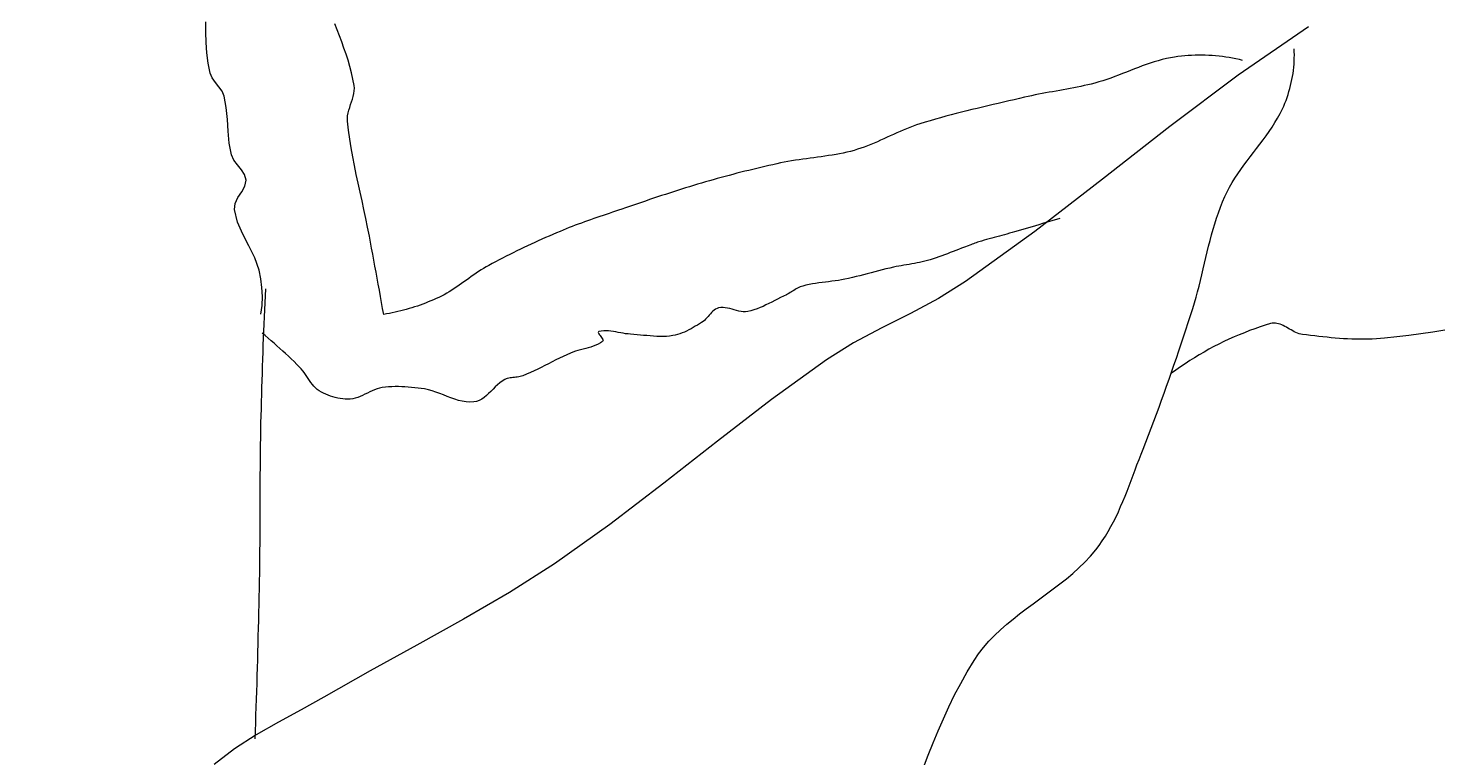
# Model space of a CAD drawing. Units: inches. Extents: x 1441 to 2460, y 1648 to 2683.
# Tile 25 of 35: x 1810 to 1840, y 2253 to 2268. Entities that reach past the tile are written whole.
import ezdxf

# ---------------------------------------------------------------- set-up
doc = ezdxf.new("R2010")
doc.units = ezdxf.units.IN
doc.layers.add('A-ANNO-DIMS', color=2, linetype='Continuous', lineweight=18)
doc.layers.add('A-FURN', color=8, linetype='Continuous', lineweight=15)
doc.styles.get("Standard").update_dxf_attribs({"font": 'arial.ttf'})
doc.dimstyles.get("Standard").update_dxf_attribs({"dimtxt": 0.18, "dimasz": 0.18, "dimexe": 0.18, "dimexo": 0.0625, "dimgap": 0.09, "dimtad": 0, "dimtih": 1, "dimtoh": 1, "dimdec": 4, "dimzin": 0, "dimdsep": 46, "dimtxsty": 'Standard', "dimcen": 0.09, "dimadec": 0, "dimazin": 0, "dimtfac": 1, "dimtdec": 4, "dimtofl": 0, "dimtmove": 0, "dimatfit": 3, "dimfxl": 1, "dimtolj": 1, "dimtzin": 0, "dimarcsym": 0})

# ---------------------------------------------------------------- blocks, each defined once
blk = doc.blocks.new('BED-DOUBLE-PLAN')
for p, q in [((4.673, 72.189), (4.668, 72.41)), ((4.68, 71.967), (4.673, 72.189)), ((7.486, 72.239), (7.436, 72.369)), ((7.535, 72.109), (7.486, 72.239)), ((28.298, 72.301), (26.791, 71.264)), ((4.695, 71.746), (4.68, 71.967)), ((7.583, 71.979), (7.535, 72.109)), ((7.63, 71.848), (7.583, 71.979)), ((4.722, 71.527), (4.695, 71.746)), ((7.675, 71.717), (7.63, 71.848)), ((7.717, 71.585), (7.675, 71.717)), ((7.755, 71.452), (7.717, 71.585)), ((25.076, 71.576), (24.99, 71.55)), ((25.162, 71.599), (25.076, 71.576)), ((25.25, 71.62), (25.162, 71.599)), ((25.337, 71.638), (25.25, 71.62)), ((25.426, 71.654), (25.337, 71.638)), ((25.498, 71.664), (25.426, 71.654)), ((25.571, 71.673), (25.498, 71.664)), ((25.644, 71.68), (25.571, 71.673)), ((25.717, 71.686), (25.644, 71.68)), ((25.79, 71.691), (25.717, 71.686)), ((25.864, 71.694), (25.79, 71.691)), ((25.938, 71.695), (25.864, 71.694)), ((26.011, 71.695), (25.938, 71.695)), ((26.085, 71.694), (26.011, 71.695)), ((26.159, 71.691), (26.085, 71.694)), ((26.233, 71.687), (26.159, 71.691)), ((26.306, 71.681), (26.233, 71.687)), ((26.379, 71.674), (26.306, 71.681)), ((26.453, 71.665), (26.379, 71.674)), ((26.525, 71.655), (26.453, 71.665)), ((26.598, 71.643), (26.525, 71.655)), ((26.67, 71.63), (26.598, 71.643)), ((26.742, 71.616), (26.67, 71.63)), ((26.814, 71.6), (26.742, 71.616)), ((26.885, 71.583), (26.814, 71.6)), ((27.985, 71.502), (27.99, 71.568)), ((27.992, 71.766), (27.99, 71.832)), ((27.99, 71.568), (27.992, 71.634)), ((27.993, 71.7), (27.992, 71.766)), ((27.992, 71.634), (27.993, 71.7)), ((4.765, 71.311), (4.722, 71.527)), ((4.809, 71.206), (4.765, 71.311)), ((7.79, 71.318), (7.755, 71.452)), ((7.821, 71.184), (7.79, 71.318)), ((24.228, 71.268), (24.144, 71.236)), ((24.313, 71.301), (24.228, 71.268)), ((24.397, 71.334), (24.313, 71.301)), ((24.481, 71.366), (24.397, 71.334)), ((24.566, 71.399), (24.481, 71.366)), ((24.65, 71.431), (24.566, 71.399)), ((24.735, 71.463), (24.65, 71.431)), ((24.819, 71.493), (24.735, 71.463)), ((24.904, 71.523), (24.819, 71.493)), ((24.99, 71.55), (24.904, 71.523)), ((27.953, 71.239), (27.964, 71.304)), ((27.964, 71.304), (27.972, 71.37)), ((27.972, 71.37), (27.98, 71.436)), ((27.98, 71.436), (27.985, 71.502)), ((4.876, 71.111), (4.809, 71.206)), ((4.95, 71.019), (4.876, 71.111)), ((5.017, 70.924), (4.95, 71.019)), ((7.846, 71.048), (7.821, 71.184)), ((7.852, 70.989), (7.846, 71.048)), ((7.85, 70.93), (7.852, 70.989)), ((23.116, 70.966), (23.041, 70.952)), ((23.192, 70.98), (23.116, 70.966)), ((23.267, 70.995), (23.192, 70.98)), ((23.342, 71.01), (23.267, 70.995)), ((23.417, 71.025), (23.342, 71.01)), ((23.492, 71.042), (23.417, 71.025)), ((23.567, 71.059), (23.492, 71.042)), ((23.641, 71.077), (23.567, 71.059)), ((23.715, 71.097), (23.641, 71.077)), ((23.802, 71.121), (23.715, 71.097)), ((23.888, 71.147), (23.802, 71.121)), ((23.974, 71.176), (23.888, 71.147)), ((24.059, 71.205), (23.974, 71.176)), ((24.144, 71.236), (24.059, 71.205)), ((26.791, 71.264), (25.327, 70.164)), ((27.877, 70.915), (27.895, 70.979)), ((27.895, 70.979), (27.912, 71.044)), ((27.912, 71.044), (27.927, 71.108)), ((27.927, 71.108), (27.941, 71.173)), ((27.941, 71.173), (27.953, 71.239)), ((5.062, 70.82), (5.017, 70.924)), ((5.108, 70.571), (5.062, 70.82)), ((7.772, 70.636), (7.792, 70.694)), ((7.792, 70.694), (7.811, 70.753)), ((7.811, 70.753), (7.828, 70.812)), ((7.828, 70.812), (7.842, 70.871)), ((7.842, 70.871), (7.85, 70.93)), ((21.648, 70.663), (21.536, 70.636)), ((21.761, 70.689), (21.648, 70.663)), ((21.874, 70.715), (21.761, 70.689)), ((21.987, 70.741), (21.874, 70.715)), ((22.1, 70.767), (21.987, 70.741)), ((22.212, 70.793), (22.1, 70.767)), ((22.287, 70.81), (22.212, 70.793)), ((22.362, 70.827), (22.287, 70.81)), ((22.437, 70.842), (22.362, 70.827)), ((22.512, 70.857), (22.437, 70.842)), ((22.588, 70.871), (22.512, 70.857)), ((22.663, 70.885), (22.588, 70.871)), ((22.739, 70.899), (22.663, 70.885)), ((22.814, 70.912), (22.739, 70.899)), ((22.89, 70.926), (22.814, 70.912)), ((22.965, 70.939), (22.89, 70.926)), ((23.041, 70.952), (22.965, 70.939)), ((27.764, 70.606), (27.789, 70.666)), ((27.789, 70.666), (27.814, 70.727)), ((27.814, 70.727), (27.836, 70.79)), ((27.836, 70.79), (27.858, 70.852)), ((27.858, 70.852), (27.877, 70.915)), ((5.131, 70.318), (5.108, 70.571)), ((7.703, 70.34), (7.708, 70.399)), ((7.708, 70.399), (7.719, 70.459)), ((7.719, 70.459), (7.734, 70.518)), ((7.734, 70.518), (7.752, 70.577)), ((7.752, 70.577), (7.772, 70.636)), ((20.525, 70.385), (20.413, 70.354)), ((20.636, 70.415), (20.525, 70.385)), ((20.748, 70.444), (20.636, 70.415)), ((20.861, 70.473), (20.748, 70.444)), ((20.973, 70.501), (20.861, 70.473)), ((21.085, 70.529), (20.973, 70.501)), ((21.198, 70.556), (21.085, 70.529)), ((21.31, 70.583), (21.198, 70.556)), ((21.423, 70.61), (21.31, 70.583)), ((21.536, 70.636), (21.423, 70.61)), ((27.633, 70.347), (27.687, 70.445)), ((27.687, 70.445), (27.736, 70.546)), ((27.736, 70.546), (27.764, 70.606)), ((5.147, 70.064), (5.131, 70.318)), ((5.17, 69.811), (5.147, 70.064)), ((7.705, 70.28), (7.703, 70.34)), ((7.727, 70.089), (7.705, 70.28)), ((7.754, 69.899), (7.727, 70.089)), ((19.544, 70.06), (19.475, 70.029)), ((19.614, 70.091), (19.544, 70.06)), ((19.684, 70.12), (19.614, 70.091)), ((19.754, 70.148), (19.684, 70.12)), ((19.825, 70.175), (19.754, 70.148)), ((19.897, 70.2), (19.825, 70.175)), ((19.969, 70.223), (19.897, 70.2)), ((20.08, 70.257), (19.969, 70.223)), ((20.191, 70.29), (20.08, 70.257)), ((20.302, 70.323), (20.191, 70.29)), ((20.413, 70.354), (20.302, 70.323)), ((25.327, 70.164), (23.883, 69.037)), ((27.387, 69.97), (27.452, 70.062)), ((27.452, 70.062), (27.515, 70.156)), ((27.515, 70.156), (27.576, 70.251)), ((27.576, 70.251), (27.633, 70.347)), ((5.217, 69.562), (5.17, 69.811)), ((7.784, 69.709), (7.754, 69.899)), ((18.848, 69.753), (18.777, 69.726)), ((18.919, 69.781), (18.848, 69.753)), ((18.989, 69.81), (18.919, 69.781)), ((19.059, 69.841), (18.989, 69.81)), ((19.128, 69.871), (19.059, 69.841)), ((19.197, 69.903), (19.128, 69.871)), ((19.267, 69.935), (19.197, 69.903)), ((19.336, 69.966), (19.267, 69.935)), ((19.405, 69.998), (19.336, 69.966)), ((19.475, 70.029), (19.405, 69.998)), ((27.184, 69.699), (27.253, 69.789)), ((27.253, 69.789), (27.321, 69.879)), ((27.321, 69.879), (27.387, 69.97)), ((5.269, 69.448), (5.217, 69.562)), ((5.347, 69.344), (5.269, 69.448)), ((7.818, 69.519), (7.784, 69.709)), ((7.855, 69.33), (7.818, 69.519)), ((17.38, 69.456), (17.301, 69.444)), ((17.459, 69.467), (17.38, 69.456)), ((17.538, 69.478), (17.459, 69.467)), ((17.618, 69.488), (17.538, 69.478)), ((17.697, 69.499), (17.618, 69.488)), ((17.777, 69.509), (17.697, 69.499)), ((17.856, 69.52), (17.777, 69.509)), ((17.935, 69.531), (17.856, 69.52)), ((18.014, 69.543), (17.935, 69.531)), ((18.093, 69.555), (18.014, 69.543)), ((18.172, 69.569), (18.093, 69.555)), ((18.25, 69.583), (18.172, 69.569)), ((18.329, 69.599), (18.25, 69.583)), ((18.407, 69.617), (18.329, 69.599)), ((18.484, 69.635), (18.407, 69.617)), ((18.561, 69.656), (18.484, 69.635)), ((18.634, 69.678), (18.561, 69.656)), ((18.706, 69.701), (18.634, 69.678)), ((18.777, 69.726), (18.706, 69.701)), ((26.978, 69.429), (27.046, 69.519)), ((27.046, 69.519), (27.115, 69.609)), ((27.115, 69.609), (27.184, 69.699)), ((5.431, 69.242), (5.347, 69.344)), ((5.5, 69.136), (5.431, 69.242)), ((7.893, 69.141), (7.855, 69.33)), ((16.05, 69.164), (15.965, 69.142)), ((16.134, 69.186), (16.05, 69.164)), ((16.219, 69.207), (16.134, 69.186)), ((16.304, 69.228), (16.219, 69.207)), ((16.389, 69.249), (16.304, 69.228)), ((16.474, 69.27), (16.389, 69.249)), ((16.559, 69.29), (16.474, 69.27)), ((16.644, 69.31), (16.559, 69.29)), ((16.73, 69.33), (16.644, 69.31)), ((16.815, 69.349), (16.73, 69.33)), ((16.901, 69.368), (16.815, 69.349)), ((16.986, 69.387), (16.901, 69.368)), ((17.064, 69.403), (16.986, 69.387)), ((17.143, 69.417), (17.064, 69.403)), ((17.222, 69.431), (17.143, 69.417)), ((17.301, 69.444), (17.222, 69.431)), ((26.718, 69.06), (26.78, 69.154)), ((26.78, 69.154), (26.844, 69.246)), ((26.844, 69.246), (26.91, 69.338)), ((26.91, 69.338), (26.978, 69.429)), ((5.44, 68.765), (5.508, 68.888)), ((5.532, 69.019), (5.5, 69.136)), ((5.508, 68.888), (5.532, 69.019)), ((7.934, 68.953), (7.893, 69.141)), ((7.975, 68.764), (7.934, 68.953)), ((14.946, 68.851), (14.86, 68.824)), ((15.032, 68.877), (14.946, 68.851)), ((15.118, 68.903), (15.032, 68.877)), ((15.204, 68.929), (15.118, 68.903)), ((15.29, 68.954), (15.204, 68.929)), ((15.375, 68.979), (15.29, 68.954)), ((15.459, 69.003), (15.375, 68.979)), ((15.543, 69.026), (15.459, 69.003)), ((15.627, 69.05), (15.543, 69.026)), ((15.711, 69.073), (15.627, 69.05)), ((15.796, 69.096), (15.711, 69.073)), ((15.88, 69.119), (15.796, 69.096)), ((15.965, 69.142), (15.88, 69.119)), ((23.883, 69.037), (22.432, 67.918)), ((26.551, 68.769), (26.603, 68.868)), ((26.603, 68.868), (26.659, 68.965)), ((26.659, 68.965), (26.718, 69.06)), ((5.296, 68.52), (5.359, 68.643)), ((5.359, 68.643), (5.44, 68.765)), ((8.017, 68.576), (7.975, 68.764)), ((8.058, 68.388), (8.017, 68.576)), ((14.006, 68.542), (13.921, 68.513)), ((14.091, 68.571), (14.006, 68.542)), ((14.176, 68.6), (14.091, 68.571)), ((14.262, 68.629), (14.176, 68.6)), ((14.347, 68.657), (14.262, 68.629)), ((14.432, 68.686), (14.347, 68.657)), ((14.518, 68.714), (14.432, 68.686)), ((14.603, 68.742), (14.518, 68.714)), ((14.689, 68.769), (14.603, 68.742)), ((14.774, 68.797), (14.689, 68.769)), ((14.86, 68.824), (14.774, 68.797)), ((26.407, 68.437), (26.453, 68.553)), ((26.453, 68.553), (26.503, 68.668)), ((26.503, 68.668), (26.551, 68.769)), ((5.281, 68.391), (5.296, 68.52)), ((5.35, 68.121), (5.281, 68.391)), ((8.098, 68.199), (8.058, 68.388)), ((13.114, 68.24), (13.048, 68.217)), ((13.181, 68.262), (13.114, 68.24)), ((13.247, 68.285), (13.181, 68.262)), ((13.314, 68.307), (13.247, 68.285)), ((13.381, 68.33), (13.314, 68.307)), ((13.447, 68.352), (13.381, 68.33)), ((13.514, 68.375), (13.447, 68.352)), ((13.58, 68.397), (13.514, 68.375)), ((13.665, 68.426), (13.58, 68.397)), ((13.75, 68.455), (13.665, 68.426)), ((13.836, 68.484), (13.75, 68.455)), ((13.921, 68.513), (13.836, 68.484)), ((26.325, 68.203), (26.365, 68.321)), ((26.365, 68.321), (26.407, 68.437)), ((5.463, 67.863), (5.35, 68.121)), ((8.137, 68.01), (8.098, 68.199)), ((8.174, 67.821), (8.137, 68.01)), ((12.324, 67.948), (12.259, 67.921)), ((12.389, 67.974), (12.324, 67.948)), ((12.454, 68.001), (12.389, 67.974)), ((12.519, 68.026), (12.454, 68.001)), ((12.585, 68.051), (12.519, 68.026)), ((12.651, 68.076), (12.585, 68.051)), ((12.717, 68.1), (12.651, 68.076)), ((12.783, 68.124), (12.717, 68.1)), ((12.849, 68.148), (12.783, 68.124)), ((12.915, 68.171), (12.849, 68.148)), ((12.981, 68.194), (12.915, 68.171)), ((13.048, 68.217), (12.981, 68.194)), ((22.073, 67.931), (21.998, 67.909)), ((22.148, 67.953), (22.073, 67.931)), ((22.223, 67.975), (22.148, 67.953)), ((22.297, 67.997), (22.223, 67.975)), ((22.372, 68.019), (22.297, 67.997)), ((22.447, 68.041), (22.372, 68.019)), ((22.521, 68.063), (22.447, 68.041)), ((22.596, 68.086), (22.521, 68.063)), ((22.671, 68.108), (22.596, 68.086)), ((22.745, 68.131), (22.671, 68.108)), ((22.82, 68.154), (22.745, 68.131)), ((22.894, 68.176), (22.82, 68.154)), ((22.969, 68.199), (22.894, 68.176)), ((26.219, 67.844), (26.252, 67.965)), ((26.252, 67.965), (26.287, 68.084)), ((26.287, 68.084), (26.325, 68.203)), ((5.593, 67.609), (5.463, 67.863)), ((8.198, 67.692), (8.174, 67.821)), ((8.222, 67.563), (8.198, 67.692)), ((11.639, 67.646), (11.562, 67.611)), ((11.716, 67.682), (11.639, 67.646)), ((11.793, 67.717), (11.716, 67.682)), ((11.87, 67.752), (11.793, 67.717)), ((11.948, 67.786), (11.87, 67.752)), ((12.025, 67.82), (11.948, 67.786)), ((12.103, 67.854), (12.025, 67.82)), ((12.181, 67.888), (12.103, 67.854)), ((12.259, 67.921), (12.181, 67.888)), ((22.432, 67.918), (20.949, 66.844)), ((21.064, 67.634), (21.036, 67.623)), ((21.092, 67.645), (21.064, 67.634)), ((21.12, 67.655), (21.092, 67.645)), ((21.149, 67.666), (21.12, 67.655)), ((21.177, 67.676), (21.149, 67.666)), ((21.206, 67.686), (21.177, 67.676)), ((21.234, 67.696), (21.206, 67.686)), ((21.263, 67.705), (21.234, 67.696)), ((21.292, 67.714), (21.263, 67.705)), ((21.346, 67.73), (21.292, 67.714)), ((21.4, 67.746), (21.346, 67.73)), ((21.454, 67.761), (21.4, 67.746)), ((21.509, 67.776), (21.454, 67.761)), ((21.563, 67.791), (21.509, 67.776)), ((21.617, 67.806), (21.563, 67.791)), ((21.672, 67.82), (21.617, 67.806)), ((21.726, 67.835), (21.672, 67.82)), ((21.781, 67.849), (21.726, 67.835)), ((21.835, 67.864), (21.781, 67.849)), ((21.89, 67.879), (21.835, 67.864)), ((21.944, 67.894), (21.89, 67.879)), ((21.998, 67.909), (21.944, 67.894)), ((26.156, 67.602), (26.187, 67.724)), ((26.187, 67.724), (26.219, 67.844)), ((5.717, 67.354), (5.593, 67.609)), ((5.81, 67.088), (5.717, 67.354)), ((8.246, 67.434), (8.222, 67.563)), ((8.27, 67.304), (8.246, 67.434)), ((11.03, 67.349), (10.955, 67.31)), ((11.105, 67.388), (11.03, 67.349)), ((11.181, 67.426), (11.105, 67.388)), ((11.257, 67.464), (11.181, 67.426)), ((11.333, 67.501), (11.257, 67.464)), ((11.409, 67.538), (11.333, 67.501)), ((11.486, 67.574), (11.409, 67.538)), ((11.562, 67.611), (11.486, 67.574)), ((20.253, 67.333), (20.191, 67.313)), ((20.315, 67.353), (20.253, 67.333)), ((20.376, 67.375), (20.315, 67.353)), ((20.437, 67.397), (20.376, 67.375)), ((20.498, 67.419), (20.437, 67.397)), ((20.558, 67.442), (20.498, 67.419)), ((20.619, 67.466), (20.558, 67.442)), ((20.679, 67.489), (20.619, 67.466)), ((20.74, 67.513), (20.679, 67.489)), ((20.8, 67.536), (20.74, 67.513)), ((20.861, 67.559), (20.8, 67.536)), ((20.922, 67.581), (20.861, 67.559)), ((20.95, 67.591), (20.922, 67.581)), ((20.979, 67.602), (20.95, 67.591)), ((21.007, 67.612), (20.979, 67.602)), ((21.036, 67.623), (21.007, 67.612)), ((26.069, 67.237), (26.098, 67.359)), ((26.098, 67.359), (26.127, 67.481)), ((26.127, 67.481), (26.156, 67.602)), ((5.849, 66.904), (5.81, 67.088)), ((8.294, 67.175), (8.27, 67.304)), ((8.318, 67.046), (8.294, 67.175)), ((8.341, 66.917), (8.318, 67.046)), ((10.461, 67.024), (10.409, 66.988)), ((10.514, 67.059), (10.461, 67.024)), ((10.567, 67.094), (10.514, 67.059)), ((10.621, 67.127), (10.567, 67.094)), ((10.675, 67.159), (10.621, 67.127)), ((10.731, 67.191), (10.675, 67.159)), ((10.805, 67.231), (10.731, 67.191)), ((10.88, 67.271), (10.805, 67.231)), ((10.955, 67.31), (10.88, 67.271)), ((18.923, 67.033), (18.843, 67.012)), ((19.003, 67.054), (18.923, 67.033)), ((19.083, 67.074), (19.003, 67.054)), ((19.163, 67.095), (19.083, 67.074)), ((19.243, 67.115), (19.163, 67.095)), ((19.324, 67.134), (19.243, 67.115)), ((19.404, 67.153), (19.324, 67.134)), ((19.46, 67.165), (19.404, 67.153)), ((19.515, 67.176), (19.46, 67.165)), ((19.571, 67.186), (19.515, 67.176)), ((19.628, 67.196), (19.571, 67.186)), ((19.684, 67.205), (19.628, 67.196)), ((19.74, 67.214), (19.684, 67.205)), ((19.796, 67.224), (19.74, 67.214)), ((19.852, 67.234), (19.796, 67.224)), ((19.908, 67.244), (19.852, 67.234)), ((19.964, 67.255), (19.908, 67.244)), ((20.019, 67.267), (19.964, 67.255)), ((20.074, 67.28), (20.019, 67.267)), ((20.129, 67.295), (20.074, 67.28)), ((20.191, 67.313), (20.129, 67.295)), ((26.012, 66.993), (26.041, 67.115)), ((26.041, 67.115), (26.069, 67.237)), ((5.873, 66.715), (5.849, 66.904)), ((8.365, 66.787), (8.341, 66.917)), ((8.388, 66.658), (8.365, 66.787)), ((10.045, 66.731), (9.992, 66.695)), ((10.097, 66.767), (10.045, 66.731)), ((10.149, 66.803), (10.097, 66.767)), ((10.201, 66.84), (10.149, 66.803)), ((10.253, 66.877), (10.201, 66.84)), ((10.305, 66.914), (10.253, 66.877)), ((10.357, 66.951), (10.305, 66.914)), ((10.409, 66.988), (10.357, 66.951)), ((17.374, 66.718), (17.347, 66.704)), ((17.402, 66.73), (17.374, 66.718)), ((17.43, 66.741), (17.402, 66.73)), ((17.459, 66.75), (17.43, 66.741)), ((17.527, 66.767), (17.459, 66.75)), ((17.596, 66.782), (17.527, 66.767)), ((17.665, 66.794), (17.596, 66.782)), ((17.734, 66.806), (17.665, 66.794)), ((17.804, 66.816), (17.734, 66.806)), ((17.874, 66.825), (17.804, 66.816)), ((17.944, 66.834), (17.874, 66.825)), ((18.014, 66.843), (17.944, 66.834)), ((18.084, 66.851), (18.014, 66.843)), ((18.154, 66.861), (18.084, 66.851)), ((18.223, 66.871), (18.154, 66.861)), ((18.293, 66.883), (18.223, 66.871)), ((18.362, 66.897), (18.293, 66.883)), ((18.443, 66.914), (18.362, 66.897)), ((18.523, 66.932), (18.443, 66.914)), ((18.603, 66.951), (18.523, 66.932)), ((18.683, 66.971), (18.603, 66.951)), ((18.764, 66.991), (18.683, 66.971)), ((18.843, 67.012), (18.764, 66.991)), ((20.949, 66.844), (20.369, 66.483)), ((25.92, 66.629), (25.952, 66.75)), ((25.952, 66.75), (25.982, 66.871)), ((25.982, 66.871), (26.012, 66.993)), ((5.881, 66.525), (5.873, 66.715)), ((5.874, 66.335), (5.881, 66.525)), ((5.939, 66.39), (5.946, 66.541)), ((5.946, 66.541), (5.953, 66.692)), ((8.412, 66.529), (8.388, 66.658)), ((8.435, 66.399), (8.412, 66.529)), ((9.493, 66.432), (9.436, 66.408)), ((9.55, 66.456), (9.493, 66.432)), ((9.607, 66.481), (9.55, 66.456)), ((9.663, 66.507), (9.607, 66.481)), ((9.72, 66.535), (9.663, 66.507)), ((9.776, 66.564), (9.72, 66.535)), ((9.831, 66.595), (9.776, 66.564)), ((9.886, 66.627), (9.831, 66.595)), ((9.939, 66.661), (9.886, 66.627)), ((9.992, 66.695), (9.939, 66.661)), ((16.859, 66.439), (16.797, 66.407)), ((16.921, 66.471), (16.859, 66.439)), ((16.983, 66.503), (16.921, 66.471)), ((17.045, 66.534), (16.983, 66.503)), ((17.108, 66.564), (17.045, 66.534)), ((17.136, 66.577), (17.108, 66.564)), ((17.163, 66.592), (17.136, 66.577)), ((17.189, 66.608), (17.163, 66.592)), ((17.215, 66.624), (17.189, 66.608)), ((17.241, 66.64), (17.215, 66.624)), ((17.268, 66.657), (17.241, 66.64)), ((17.294, 66.673), (17.268, 66.657)), ((17.32, 66.689), (17.294, 66.673)), ((17.347, 66.704), (17.32, 66.689)), ((20.369, 66.483), (19.765, 66.161)), ((25.852, 66.388), (25.887, 66.508)), ((25.887, 66.508), (25.92, 66.629)), ((5.851, 66.148), (5.874, 66.335)), ((5.926, 66.088), (5.932, 66.239)), ((5.932, 66.239), (5.939, 66.39)), ((8.458, 66.27), (8.435, 66.399)), ((8.481, 66.141), (8.458, 66.27)), ((8.542, 66.151), (8.481, 66.141)), ((8.603, 66.163), (8.542, 66.151)), ((8.664, 66.175), (8.603, 66.163)), ((8.725, 66.188), (8.664, 66.175)), ((8.785, 66.202), (8.725, 66.188)), ((8.845, 66.216), (8.785, 66.202)), ((8.905, 66.232), (8.845, 66.216)), ((8.965, 66.248), (8.905, 66.232)), ((9.025, 66.266), (8.965, 66.248)), ((9.085, 66.284), (9.025, 66.266)), ((9.144, 66.303), (9.085, 66.284)), ((9.203, 66.322), (9.144, 66.303)), ((9.262, 66.342), (9.203, 66.322)), ((9.32, 66.364), (9.262, 66.342)), ((9.378, 66.386), (9.32, 66.364)), ((9.436, 66.408), (9.378, 66.386)), ((15.455, 66.127), (15.43, 66.097)), ((15.481, 66.156), (15.455, 66.127)), ((15.506, 66.183), (15.481, 66.156)), ((15.533, 66.209), (15.506, 66.183)), ((15.561, 66.233), (15.533, 66.209)), ((15.591, 66.253), (15.561, 66.233)), ((15.623, 66.268), (15.591, 66.253)), ((15.658, 66.28), (15.623, 66.268)), ((15.705, 66.287), (15.658, 66.28)), ((15.752, 66.289), (15.705, 66.287)), ((15.8, 66.285), (15.752, 66.289)), ((15.848, 66.277), (15.8, 66.285)), ((15.896, 66.266), (15.848, 66.277)), ((15.945, 66.253), (15.896, 66.266)), ((15.993, 66.239), (15.945, 66.253)), ((16.042, 66.226), (15.993, 66.239)), ((16.09, 66.215), (16.042, 66.226)), ((16.138, 66.206), (16.09, 66.215)), ((16.186, 66.2), (16.138, 66.206)), ((16.234, 66.2), (16.186, 66.2)), ((16.282, 66.206), (16.234, 66.2)), ((16.349, 66.221), (16.282, 66.206)), ((16.415, 66.24), (16.349, 66.221)), ((16.48, 66.263), (16.415, 66.24)), ((16.545, 66.288), (16.48, 66.263)), ((16.609, 66.315), (16.545, 66.288)), ((16.672, 66.344), (16.609, 66.315)), ((16.734, 66.375), (16.672, 66.344)), ((16.797, 66.407), (16.734, 66.375)), ((19.765, 66.161), (19.153, 65.853)), ((25.716, 65.966), (25.765, 66.117)), ((25.765, 66.117), (25.815, 66.269)), ((25.815, 66.269), (25.852, 66.388)), ((5.913, 65.785), (5.92, 65.936)), ((5.92, 65.936), (5.926, 66.088)), ((15.019, 65.81), (14.972, 65.786)), ((15.066, 65.835), (15.019, 65.81)), ((15.112, 65.861), (15.066, 65.835)), ((15.157, 65.887), (15.112, 65.861)), ((15.202, 65.914), (15.157, 65.887)), ((15.247, 65.942), (15.202, 65.914)), ((15.292, 65.969), (15.247, 65.942)), ((15.323, 65.99), (15.292, 65.969)), ((15.351, 66.014), (15.323, 65.99)), ((15.379, 66.04), (15.351, 66.014)), ((15.405, 66.068), (15.379, 66.04)), ((15.43, 66.097), (15.405, 66.068)), ((19.153, 65.853), (18.549, 65.531)), ((25.616, 65.662), (25.666, 65.814)), ((25.666, 65.814), (25.716, 65.966)), ((27.145, 65.835), (27.033, 65.794)), ((27.257, 65.874), (27.145, 65.835)), ((27.37, 65.911), (27.257, 65.874)), ((27.484, 65.946), (27.37, 65.911)), ((27.519, 65.953), (27.484, 65.946)), ((27.553, 65.957), (27.519, 65.953)), ((27.587, 65.955), (27.553, 65.957)), ((27.62, 65.951), (27.587, 65.955)), ((27.654, 65.942), (27.62, 65.951)), ((27.688, 65.931), (27.654, 65.942)), ((27.721, 65.918), (27.688, 65.931)), ((27.755, 65.902), (27.721, 65.918)), ((27.788, 65.885), (27.755, 65.902)), ((27.822, 65.867), (27.788, 65.885)), ((27.855, 65.847), (27.822, 65.867)), ((27.889, 65.828), (27.855, 65.847)), ((27.923, 65.809), (27.889, 65.828)), ((27.957, 65.79), (27.923, 65.809)), ((5.943, 65.687), (5.879, 65.74)), ((5.902, 65.483), (5.908, 65.634)), ((5.908, 65.634), (5.913, 65.785)), ((6.006, 65.633), (5.943, 65.687)), ((6.07, 65.579), (6.006, 65.633)), ((6.133, 65.525), (6.07, 65.579)), ((6.195, 65.47), (6.133, 65.525)), ((13.075, 65.503), (13.024, 65.48)), ((13.123, 65.53), (13.075, 65.503)), ((13.081, 65.766), (13.078, 65.756)), ((13.078, 65.756), (13.081, 65.742)), ((13.093, 65.773), (13.081, 65.766)), ((13.081, 65.742), (13.09, 65.726)), ((13.09, 65.726), (13.103, 65.707)), ((13.144, 65.784), (13.093, 65.773)), ((13.103, 65.707), (13.118, 65.687)), ((13.118, 65.687), (13.135, 65.667)), ((13.169, 65.562), (13.123, 65.53)), ((13.135, 65.667), (13.151, 65.646)), ((13.195, 65.789), (13.144, 65.784)), ((13.151, 65.646), (13.164, 65.626)), ((13.164, 65.626), (13.175, 65.606)), ((13.179, 65.574), (13.169, 65.562)), ((13.175, 65.606), (13.18, 65.589)), ((13.18, 65.589), (13.179, 65.574)), ((13.247, 65.791), (13.195, 65.789)), ((13.298, 65.788), (13.247, 65.791)), ((13.35, 65.783), (13.298, 65.788)), ((13.403, 65.776), (13.35, 65.783)), ((13.455, 65.767), (13.403, 65.776)), ((13.508, 65.757), (13.455, 65.767)), ((13.56, 65.747), (13.508, 65.757)), ((13.613, 65.738), (13.56, 65.747)), ((13.665, 65.729), (13.613, 65.738)), ((13.718, 65.723), (13.665, 65.729)), ((13.77, 65.718), (13.718, 65.723)), ((13.84, 65.714), (13.77, 65.718)), ((13.91, 65.708), (13.84, 65.714)), ((13.98, 65.701), (13.91, 65.708)), ((14.05, 65.694), (13.98, 65.701)), ((14.12, 65.688), (14.05, 65.694)), ((14.19, 65.681), (14.12, 65.688)), ((14.26, 65.676), (14.19, 65.681)), ((14.33, 65.672), (14.26, 65.676)), ((14.399, 65.669), (14.33, 65.672)), ((14.469, 65.669), (14.399, 65.669)), ((14.539, 65.672), (14.469, 65.669)), ((14.608, 65.678), (14.539, 65.672)), ((14.677, 65.687), (14.608, 65.678)), ((14.728, 65.697), (14.677, 65.687)), ((14.778, 65.71), (14.728, 65.697)), ((14.828, 65.726), (14.778, 65.71)), ((14.876, 65.744), (14.828, 65.726)), ((14.924, 65.764), (14.876, 65.744)), ((14.972, 65.786), (14.924, 65.764)), ((18.549, 65.531), (17.968, 65.172)), ((25.515, 65.359), (25.566, 65.51)), ((25.566, 65.51), (25.616, 65.662)), ((26.375, 65.506), (26.269, 65.452)), ((26.483, 65.559), (26.375, 65.506)), ((26.591, 65.61), (26.483, 65.559)), ((26.7, 65.659), (26.591, 65.61)), ((26.81, 65.706), (26.7, 65.659)), ((26.921, 65.751), (26.81, 65.706)), ((27.033, 65.794), (26.921, 65.751)), ((27.991, 65.772), (27.957, 65.79)), ((28.025, 65.756), (27.991, 65.772)), ((28.06, 65.741), (28.025, 65.756)), ((28.094, 65.729), (28.06, 65.741)), ((28.13, 65.72), (28.094, 65.729)), ((28.165, 65.713), (28.13, 65.72)), ((28.253, 65.702), (28.165, 65.713)), ((28.34, 65.691), (28.253, 65.702)), ((28.428, 65.681), (28.34, 65.691)), ((28.516, 65.67), (28.428, 65.681)), ((28.604, 65.661), (28.516, 65.67)), ((28.692, 65.652), (28.604, 65.661)), ((28.78, 65.643), (28.692, 65.652)), ((28.869, 65.635), (28.78, 65.643)), ((28.957, 65.628), (28.869, 65.635)), ((29.045, 65.622), (28.957, 65.628)), ((29.133, 65.617), (29.045, 65.622)), ((29.222, 65.613), (29.133, 65.617)), ((29.31, 65.611), (29.222, 65.613)), ((29.398, 65.609), (29.31, 65.611)), ((29.487, 65.609), (29.398, 65.609)), ((29.575, 65.61), (29.487, 65.609)), ((29.663, 65.613), (29.575, 65.61)), ((29.751, 65.618), (29.663, 65.613)), ((29.839, 65.624), (29.751, 65.618)), ((29.927, 65.632), (29.839, 65.624)), ((30.186, 65.66), (29.927, 65.632)), ((30.444, 65.692), (30.186, 65.66)), ((30.702, 65.727), (30.444, 65.692)), ((30.96, 65.765), (30.702, 65.727)), ((31.218, 65.805), (30.96, 65.765)), ((5.891, 65.181), (5.896, 65.332)), ((5.896, 65.332), (5.902, 65.483)), ((6.257, 65.414), (6.195, 65.47)), ((6.319, 65.358), (6.257, 65.414)), ((6.38, 65.302), (6.319, 65.358)), ((6.44, 65.245), (6.38, 65.302)), ((6.501, 65.188), (6.44, 65.245)), ((12.246, 65.204), (12.168, 65.166)), ((12.324, 65.242), (12.246, 65.204)), ((12.403, 65.279), (12.324, 65.242)), ((12.482, 65.314), (12.403, 65.279)), ((12.535, 65.335), (12.482, 65.314)), ((12.588, 65.353), (12.535, 65.335)), ((12.643, 65.369), (12.588, 65.353)), ((12.698, 65.384), (12.643, 65.369)), ((12.754, 65.398), (12.698, 65.384)), ((12.809, 65.412), (12.754, 65.398)), ((12.864, 65.426), (12.809, 65.412)), ((12.919, 65.442), (12.864, 65.426)), ((12.972, 65.46), (12.919, 65.442)), ((13.024, 65.48), (12.972, 65.46)), ((25.413, 65.056), (25.464, 65.207)), ((25.464, 65.207), (25.515, 65.359)), ((25.853, 65.215), (25.752, 65.152)), ((25.955, 65.277), (25.853, 65.215)), ((26.059, 65.337), (25.955, 65.277)), ((26.163, 65.395), (26.059, 65.337)), ((26.269, 65.452), (26.163, 65.395)), ((5.881, 64.878), (5.886, 65.029)), ((5.886, 65.029), (5.891, 65.181)), ((6.56, 65.13), (6.501, 65.188)), ((6.619, 65.071), (6.56, 65.13)), ((6.678, 65.013), (6.619, 65.071)), ((6.713, 64.975), (6.678, 65.013)), ((6.745, 64.936), (6.713, 64.975)), ((6.776, 64.895), (6.745, 64.936)), ((11.702, 64.932), (11.623, 64.896)), ((11.78, 64.97), (11.702, 64.932)), ((11.858, 65.008), (11.78, 64.97)), ((11.935, 65.048), (11.858, 65.008)), ((12.013, 65.087), (11.935, 65.048)), ((12.09, 65.127), (12.013, 65.087)), ((12.168, 65.166), (12.09, 65.127)), ((17.968, 65.172), (16.787, 64.32)), ((25.308, 64.754), (25.361, 64.905)), ((25.456, 64.951), (25.36, 64.881)), ((25.361, 64.905), (25.413, 65.056)), ((25.553, 65.02), (25.456, 64.951)), ((25.652, 65.087), (25.553, 65.02)), ((25.752, 65.152), (25.652, 65.087)), ((5.872, 64.576), (5.876, 64.727)), ((5.876, 64.727), (5.881, 64.878)), ((6.805, 64.853), (6.776, 64.895)), ((6.834, 64.81), (6.805, 64.853)), ((6.863, 64.767), (6.834, 64.81)), ((6.892, 64.724), (6.863, 64.767)), ((6.922, 64.683), (6.892, 64.724)), ((6.953, 64.643), (6.922, 64.683)), ((6.985, 64.605), (6.953, 64.643)), ((7.021, 64.569), (6.985, 64.605)), ((8.657, 64.594), (8.587, 64.59)), ((8.727, 64.596), (8.657, 64.594)), ((8.797, 64.596), (8.727, 64.596)), ((8.867, 64.594), (8.797, 64.596)), ((8.937, 64.591), (8.867, 64.594)), ((10.919, 64.633), (10.871, 64.588)), ((10.969, 64.676), (10.919, 64.633)), ((11.02, 64.714), (10.969, 64.676)), ((11.074, 64.746), (11.02, 64.714)), ((11.102, 64.759), (11.074, 64.746)), ((11.13, 64.769), (11.102, 64.759)), ((11.16, 64.777), (11.13, 64.769)), ((11.19, 64.782), (11.16, 64.777)), ((11.22, 64.787), (11.19, 64.782)), ((11.251, 64.79), (11.22, 64.787)), ((11.282, 64.793), (11.251, 64.79)), ((11.313, 64.796), (11.282, 64.793)), ((11.344, 64.799), (11.313, 64.796)), ((11.375, 64.803), (11.344, 64.799)), ((11.405, 64.809), (11.375, 64.803)), ((11.435, 64.817), (11.405, 64.809)), ((11.463, 64.827), (11.435, 64.817)), ((11.544, 64.86), (11.463, 64.827)), ((11.623, 64.896), (11.544, 64.86)), ((25.202, 64.453), (25.256, 64.603)), ((25.256, 64.603), (25.308, 64.754)), ((5.863, 64.273), (5.868, 64.425)), ((5.868, 64.425), (5.872, 64.576)), ((7.058, 64.536), (7.021, 64.569)), ((7.099, 64.507), (7.058, 64.536)), ((7.145, 64.48), (7.099, 64.507)), ((7.192, 64.455), (7.145, 64.48)), ((7.24, 64.432), (7.192, 64.455)), ((7.289, 64.411), (7.24, 64.432)), ((7.34, 64.392), (7.289, 64.411)), ((7.391, 64.375), (7.34, 64.392)), ((7.443, 64.361), (7.391, 64.375)), ((7.496, 64.349), (7.443, 64.361)), ((7.549, 64.339), (7.496, 64.349)), ((7.602, 64.333), (7.549, 64.339)), ((7.655, 64.328), (7.602, 64.333)), ((7.708, 64.327), (7.655, 64.328)), ((7.761, 64.328), (7.708, 64.327)), ((7.817, 64.334), (7.761, 64.328)), ((7.871, 64.346), (7.817, 64.334)), ((7.924, 64.363), (7.871, 64.346)), ((7.976, 64.383), (7.924, 64.363)), ((8.028, 64.406), (7.976, 64.383)), ((8.08, 64.431), (8.028, 64.406)), ((8.131, 64.457), (8.08, 64.431)), ((8.183, 64.483), (8.131, 64.457)), ((8.234, 64.508), (8.183, 64.483)), ((8.286, 64.53), (8.234, 64.508)), ((8.339, 64.55), (8.286, 64.53)), ((8.393, 64.565), (8.339, 64.55)), ((8.448, 64.576), (8.393, 64.565)), ((8.518, 64.584), (8.448, 64.576)), ((8.587, 64.59), (8.518, 64.584)), ((9.007, 64.586), (8.937, 64.591)), ((9.077, 64.58), (9.007, 64.586)), ((9.147, 64.573), (9.077, 64.58)), ((9.217, 64.564), (9.147, 64.573)), ((9.286, 64.555), (9.217, 64.564)), ((9.355, 64.545), (9.286, 64.555)), ((9.438, 64.528), (9.355, 64.545)), ((9.52, 64.506), (9.438, 64.528)), ((9.601, 64.479), (9.52, 64.506)), ((9.682, 64.449), (9.601, 64.479)), ((9.762, 64.417), (9.682, 64.449)), ((9.842, 64.385), (9.762, 64.417)), ((9.922, 64.354), (9.842, 64.385)), ((10.003, 64.325), (9.922, 64.354)), ((10.083, 64.301), (10.003, 64.325)), ((10.164, 64.281), (10.083, 64.301)), ((10.528, 64.301), (10.471, 64.28)), ((10.582, 64.33), (10.528, 64.301)), ((10.633, 64.365), (10.582, 64.33)), ((10.682, 64.405), (10.633, 64.365)), ((10.73, 64.448), (10.682, 64.405)), ((10.777, 64.494), (10.73, 64.448)), ((10.824, 64.541), (10.777, 64.494)), ((10.871, 64.588), (10.824, 64.541)), ((16.787, 64.32), (15.632, 63.429)), ((25.093, 64.152), (25.148, 64.303)), ((25.148, 64.303), (25.202, 64.453)), ((5.856, 63.971), (5.86, 64.122)), ((5.86, 64.122), (5.863, 64.273)), ((10.246, 64.268), (10.164, 64.281)), ((10.328, 64.264), (10.246, 64.268)), ((10.411, 64.268), (10.328, 64.264)), ((10.471, 64.28), (10.411, 64.268)), ((24.982, 63.853), (25.038, 64.003)), ((25.038, 64.003), (25.093, 64.152)), ((5.849, 63.668), (5.852, 63.82)), ((5.852, 63.82), (5.856, 63.971)), ((24.868, 63.555), (24.925, 63.704)), ((24.925, 63.704), (24.982, 63.853)), ((5.843, 63.345), (5.846, 63.507)), ((5.846, 63.507), (5.849, 63.668)), ((15.632, 63.429), (14.485, 62.528)), ((24.751, 63.258), (24.81, 63.406)), ((24.81, 63.406), (24.868, 63.555)), ((5.839, 63.021), (5.841, 63.183)), ((5.841, 63.183), (5.843, 63.345)), ((24.664, 63.035), (24.707, 63.147)), ((24.707, 63.147), (24.751, 63.258)), ((5.837, 62.698), (5.838, 62.86)), ((5.838, 62.86), (5.839, 63.021)), ((24.537, 62.697), (24.579, 62.81)), ((24.579, 62.81), (24.621, 62.923)), ((24.621, 62.923), (24.664, 63.035)), ((5.835, 62.374), (5.836, 62.536)), ((5.836, 62.536), (5.837, 62.698)), ((14.485, 62.528), (13.327, 61.643)), ((24.409, 62.359), (24.452, 62.471)), ((24.452, 62.471), (24.495, 62.584)), ((24.495, 62.584), (24.537, 62.697)), ((5.834, 62.051), (5.835, 62.213)), ((5.835, 62.213), (5.835, 62.374)), ((24.319, 62.135), (24.364, 62.247)), ((24.364, 62.247), (24.409, 62.359)), ((5.833, 61.727), (5.834, 61.889)), ((5.834, 61.889), (5.834, 62.051)), ((24.172, 61.808), (24.223, 61.916)), ((24.223, 61.916), (24.271, 62.025)), ((24.271, 62.025), (24.319, 62.135)), ((5.832, 61.404), (5.833, 61.565)), ((5.833, 61.565), (5.833, 61.727)), ((13.327, 61.643), (12.139, 60.8)), ((24.004, 61.492), (24.063, 61.596)), ((24.063, 61.596), (24.119, 61.701)), ((24.119, 61.701), (24.172, 61.808)), ((5.831, 61.242), (5.832, 61.404)), ((23.809, 61.195), (23.878, 61.292)), ((23.878, 61.292), (23.943, 61.391)), ((23.943, 61.391), (24.004, 61.492)), ((5.828, 60.918), (5.83, 61.08)), ((5.83, 61.08), (5.831, 61.242)), ((23.502, 60.838), (23.623, 60.966)), ((23.623, 60.966), (23.737, 61.1)), ((23.737, 61.1), (23.809, 61.195)), ((5.824, 60.595), (5.826, 60.757)), ((5.826, 60.757), (5.828, 60.918)), ((12.139, 60.8), (11.176, 60.189)), ((23.244, 60.596), (23.376, 60.715)), ((23.376, 60.715), (23.502, 60.838)), ((5.818, 60.264), (5.821, 60.433)), ((5.821, 60.433), (5.824, 60.595)), ((22.826, 60.262), (22.968, 60.371)), ((22.968, 60.371), (23.108, 60.482)), ((23.108, 60.482), (23.244, 60.596)), ((5.811, 59.926), (5.815, 60.095)), ((5.815, 60.095), (5.818, 60.264)), ((11.176, 60.189), (10.189, 59.615)), ((22.393, 59.942), (22.538, 60.048)), ((22.538, 60.048), (22.683, 60.154)), ((22.683, 60.154), (22.826, 60.262)), ((5.803, 59.588), (5.807, 59.757)), ((5.807, 59.757), (5.811, 59.926)), ((22.107, 59.727), (22.249, 59.835)), ((22.249, 59.835), (22.393, 59.942)), ((5.799, 59.419), (5.803, 59.588)), ((10.189, 59.615), (9.189, 59.061)), ((21.698, 59.388), (21.83, 59.504)), ((21.83, 59.504), (21.967, 59.617)), ((21.967, 59.617), (22.107, 59.727)), ((5.791, 59.081), (5.795, 59.25)), ((5.795, 59.25), (5.799, 59.419)), ((21.335, 59.01), (21.449, 59.141)), ((21.449, 59.141), (21.571, 59.267)), ((21.571, 59.267), (21.698, 59.388)), ((5.782, 58.743), (5.786, 58.912)), ((5.786, 58.912), (5.791, 59.081)), ((9.189, 59.061), (8.189, 58.51)), ((21.129, 58.727), (21.227, 58.872)), ((21.227, 58.872), (21.335, 59.01)), ((5.772, 58.406), (5.777, 58.575)), ((5.777, 58.575), (5.782, 58.743)), ((20.982, 58.486), (21.129, 58.727)), ((5.761, 58.068), (5.767, 58.237)), ((5.767, 58.237), (5.772, 58.406)), ((8.189, 58.51), (7.197, 57.943)), ((20.714, 57.991), (20.844, 58.24)), ((20.844, 58.24), (20.982, 58.486)), ((5.756, 57.899), (5.761, 58.068)), ((7.197, 57.943), (6.716, 57.672)), ((20.59, 57.739), (20.714, 57.991)), ((5.744, 57.561), (5.75, 57.73)), ((5.75, 57.73), (5.756, 57.899)), ((6.716, 57.672), (6.229, 57.407)), ((20.473, 57.483), (20.59, 57.739)), ((5.732, 57.223), (5.738, 57.392)), ((5.738, 57.392), (5.744, 57.561)), ((6.229, 57.407), (5.748, 57.134)), ((20.361, 57.224), (20.473, 57.483)), ((5.748, 57.134), (5.285, 56.837)), ((5.726, 57.054), (5.732, 57.223)), ((20.254, 56.963), (20.361, 57.224)), ((5.285, 56.837), (4.851, 56.5)), ((20.15, 56.7), (20.254, 56.963)), ((20.05, 56.435), (20.15, 56.7))]:
    blk.add_line(p, q)
blk = doc.blocks.new('*D67')
at = {"layer": 'A-ANNO-DIMS', "color": 0, "lineweight": -2, "transparency": 16777216}
for p, q in [((1889.448, 2298.695), (1916.216, 2298.695)), ((1916.036, 2298.515), (1916.036, 2055.938)), ((1916.036, 1812.997), (1916.036, 2055.574)), ((1758.224, 1812.817), (1916.216, 1812.817))]:
    blk.add_line(p, q, dxfattribs=at)
at = {"layer": 'A-ANNO-DIMS', "color": 0, "transparency": 16777216}
for points in [[(1916.006, 2298.515), (1916.066, 2298.515), (1916.036, 2298.695)], [(1916.006, 1812.997), (1916.066, 1812.997), (1916.036, 1812.817)]]:
    blk.add_solid(points, dxfattribs=at)
at = {"layer": 'Defpoints', "color": 0, "transparency": 16777216}
for p in [(1889.386, 2298.695), (1916.036, 2298.695), (1758.161, 1812.817)]:
    blk.add_point(p, dxfattribs=at)
at = {"layer": 'A-ANNO-DIMS', "color": 0, "transparency": 16777216, "insert": (1916.036, 2055.756), "char_height": 0.18, "attachment_point": 5}
blk.add_mtext('\\A1;485.9', dxfattribs=at)

msp = doc.modelspace()

# ---------------------------------------------------------------- block references
at = {"layer": 'A-FURN'}
msp.add_blockref('BED-DOUBLE-PLAN', (1809.2, 2196.18), dxfattribs=at)

# ---------------------------------------------------------------- dimensions: what is measured, and where the dimension line sits
at = {"layer": 'A-ANNO-DIMS'}
dim = msp.add_linear_dim(base=(1916.0359, 2298.6952), p1=(1758.1615, 1812.8171), p2=(1889.3859, 2298.6952), angle=90, dimstyle='Standard', override={"dimdec": 1, "dimlfac": 1, "dimrnd": 0, "dimzin": 0, "dimdsep": 46, "dimlunit": 2}, dxfattribs=at)
dim.commit()
dim.dimension.update_dxf_attribs({"geometry": '*D67', "text_midpoint": (1916.0359, 2055.7561)})

doc.saveas('drawing.dxf')
